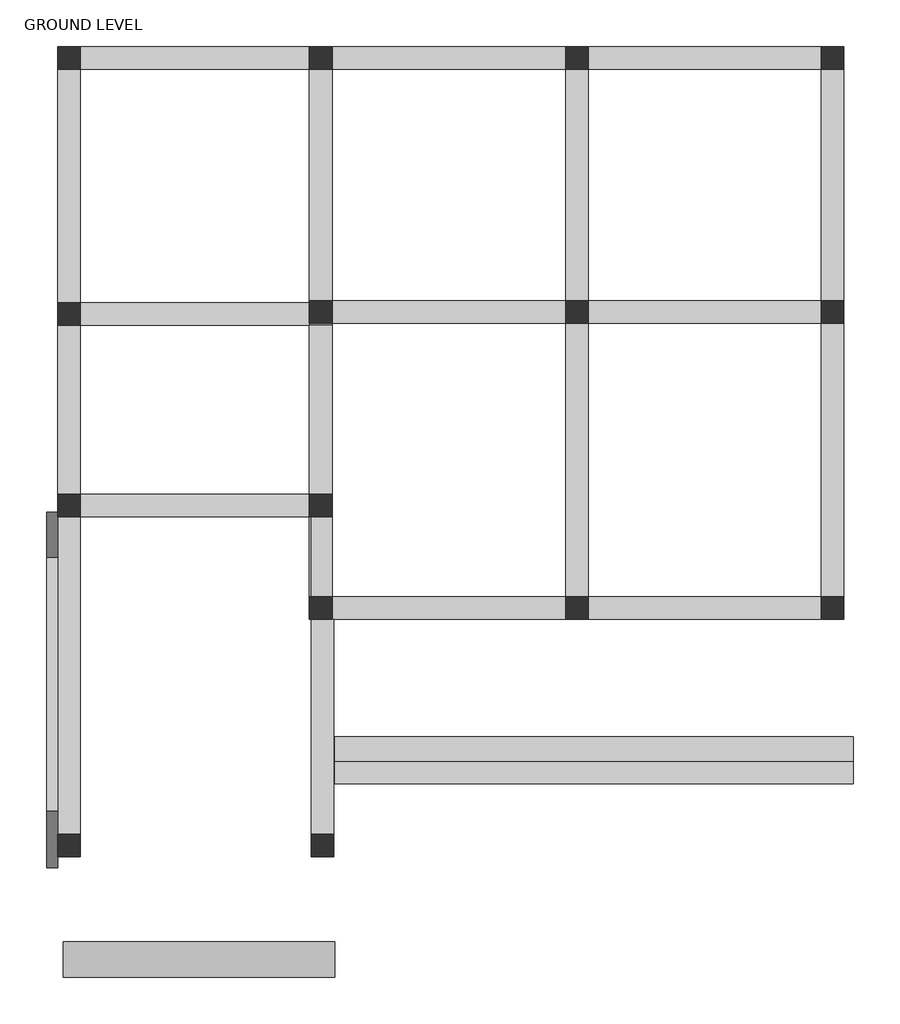
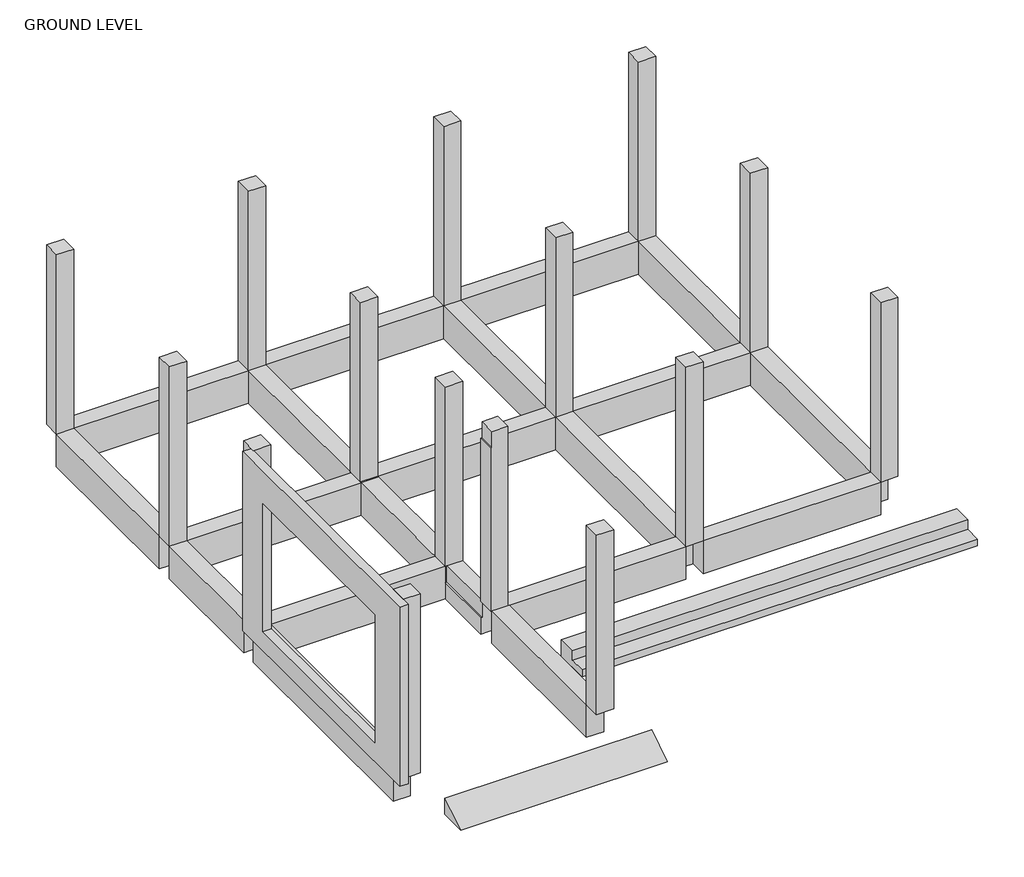
# One storey: 20 beams, 15 columns, 3 proxies.
"""IFC4 building model written with IfcOpenShell, lengths in millimetres."""

from ifc_helpers import new_model, si_unit, frame, origin, origin_with_axes, place, context, project, spatial, polyline, outline, extrude, faceted_brep, transform, mapped, element, save
from components import proxy_c6281e4c, generic_models_12_generic_models_12_89349366, generic_models_13_generic_models_13_4f71b6b5

model = new_model("IFC4")

# Units and contexts
model_context = context("Model", 3, world=origin())
ifc_project = project(units=[si_unit("LENGTHUNIT", "METRE", prefix="MILLI")], contexts=[model_context])

# Site, building, storey
site = spatial("IfcSite", under=ifc_project)
building = spatial("IfcBuilding", under=site)
storey = spatial("IfcBuildingStorey", under=building, Name="GROUND LEVEL", Elevation=0.0)

# Beams
placement = place(None, origin())
element("IfcBeam", 1, ObjectType="Concrete-Rectangular Beam : 12 x 24", at=placement, inside=storey, context=model_context, shape_type="Brep", body=[
    faceted_brep([(-11643.8293601, -6018.4747117, 0.0), (-11339.0293601, -6018.4747117, 0.0), (-11339.0293601, -2868.8747117, 0.0), (-11643.8293601, -2868.8747117, 0.0), (-11643.8293601, -6018.4747117, -609.6), (-11643.8293601, -2868.8747117, -609.6), (-11339.0293601, -6018.4747117, -609.6), (-11339.0293601, -2868.8747117, -609.6), (-11339.0293601, -6018.4747117, -304.8), (-11339.0293601, -2868.8747117, -304.8)], [[[0, 1, 2, 3]], [[4, 0, 3, 5]], [[6, 4, 5, 7]], [[1, 8, 6, 7, 9, 2]], [[2, 9, 7, 5, 3]], [[1, 0, 4, 6, 8]]]),
])
element("IfcBeam", 2, ObjectType="Concrete-Rectangular Beam : 12 x 24", at=placement, inside=storey, context=model_context, shape_type="Brep", body=[
    faceted_brep([(-8251.5270642, -2868.8747117, 0.0), (-8251.5270642, -2564.0747117, 0.0), (-11339.0293601, -2564.0747117, 0.0), (-11339.0293601, -2868.8747117, 0.0), (-8251.5270642, -2868.8747117, -609.6), (-8251.5270642, -2868.8747117, -304.8), (-11339.0293601, -2868.8747117, -304.8), (-11339.0293601, -2868.8747117, -609.6), (-8251.5270642, -2564.0747117, -609.6), (-11339.0293601, -2564.0747117, -609.6)], [[[0, 1, 2, 3]], [[4, 5, 0, 3, 6, 7]], [[8, 4, 7, 9]], [[1, 8, 9, 2]], [[2, 9, 7, 6, 3]], [[1, 0, 5, 4, 8]]]),
])
element("IfcBeam", 3, ObjectType="Concrete-Rectangular Beam : 12 x 24", at=placement, inside=storey, context=model_context, shape_type="Brep", body=[
    faceted_brep([(-4797.1270642, -2868.8747117, 0.0), (-4797.1270642, -2564.0747117, 0.0), (-7946.7270642, -2564.0747117, 0.0), (-7946.7270642, -2868.8747117, 0.0), (-4797.1270642, -2868.8747117, -609.6), (-4797.1270642, -2868.8747117, -304.8), (-7946.7270642, -2868.8747117, -304.8), (-7946.7270642, -2868.8747117, -609.6), (-4797.1270642, -2564.0747117, -609.6), (-7946.7270642, -2564.0747117, -609.6)], [[[0, 1, 2, 3]], [[4, 5, 0, 3, 6, 7]], [[8, 4, 7, 9]], [[1, 8, 9, 2]], [[2, 9, 7, 6, 3]], [[1, 0, 5, 4, 8]]]),
])
element("IfcBeam", 4, ObjectType="Concrete-Rectangular Beam : 12 x 24", at=placement, inside=storey, context=model_context, shape_type="Brep", body=[
    faceted_brep([(-1351.9658472, -2868.8747117, 0.0), (-1351.9658472, -2564.0747117, 0.0), (-4492.3270642, -2564.0747117, 0.0), (-4492.3270642, -2868.8747117, 0.0), (-1351.9658472, -2868.8747117, -609.6), (-1351.9658472, -2868.8747117, -304.8), (-4492.3270642, -2868.8747117, -304.8), (-4492.3270642, -2868.8747117, -609.6), (-1351.9658472, -2564.0747117, -609.6), (-4492.3270642, -2564.0747117, -609.6)], [[[0, 1, 2, 3]], [[4, 5, 0, 3, 6, 7]], [[8, 4, 7, 9]], [[1, 8, 9, 2]], [[2, 9, 7, 6, 3]], [[1, 0, 5, 4, 8]]]),
])
element("IfcBeam", 5, ObjectType="Concrete-Rectangular Beam : 12 x 24", at=placement, inside=storey, context=model_context, shape_type="Brep", body=[
    faceted_brep([(-1351.9658472, -5993.0747117, 0.0), (-1047.1658472, -5993.0747117, 0.0), (-1047.1658472, -2868.8747117, 0.0), (-1351.9658472, -2868.8747117, 0.0), (-1351.9658472, -5993.0747117, -609.6), (-1351.9658472, -5993.0747117, -304.8), (-1351.9658472, -2868.8747117, -304.8), (-1351.9658472, -2868.8747117, -609.6), (-1047.1658472, -5993.0747117, -609.6), (-1047.1658472, -2868.8747117, -609.6)], [[[0, 1, 2, 3]], [[4, 5, 0, 3, 6, 7]], [[8, 4, 7, 9]], [[1, 8, 9, 2]], [[2, 9, 7, 6, 3]], [[1, 0, 5, 4, 8]]]),
])
element("IfcBeam", 6, ObjectType="Concrete-Rectangular Beam : 12 x 24", at=placement, inside=storey, context=model_context, shape_type="Brep", body=[
    faceted_brep([(-7946.7270642, -2868.8747117, 0.0), (-8251.5270642, -2868.8747117, 0.0), (-8251.5270642, -5993.0747117, 0.0), (-7946.7270642, -5993.0747117, 0.0), (-8251.5270642, -2868.8747117, -304.8), (-8251.5270642, -2868.8747117, -609.6), (-8251.5270642, -5993.0747117, -609.6), (-7946.7270642, -2868.8747117, -609.6), (-7946.7270642, -5993.0747117, -609.6), (-7946.7270642, -2868.8747117, -304.8), (-7946.7270642, -5993.0747117, -304.8)], [[[0, 1, 2, 3]], [[1, 4, 5, 6, 2]], [[5, 7, 8, 6]], [[7, 9, 0, 3, 10, 8]], [[0, 9, 7, 5, 4, 1]], [[3, 2, 6, 8, 10]]]),
    faceted_brep([(-7946.7270642, -6323.2747117, 0.0), (-8251.5270642, -6323.2747117, 0.0), (-8251.5270642, -6323.2747117, -609.6), (-7946.7270642, -6323.2747117, -609.6), (-8251.5270642, -6297.8747117, 0.0), (-7946.7270642, -6297.8747117, 0.0), (-7946.7270642, -6297.8747117, -609.6), (-8251.5270642, -6297.8747117, -609.6)], [[[0, 1, 2, 3]], [[4, 5, 6, 7]], [[1, 0, 5, 4]], [[2, 1, 4, 7]], [[3, 2, 7, 6]], [[0, 3, 6, 5]]]),
])
element("IfcBeam", 7, ObjectType="Concrete-Rectangular Beam : 12 x 24", at=placement, inside=storey, context=model_context, shape_type="Brep", body=[
    faceted_brep([(-1351.9658472, -9984.0050402, 0.0), (-1047.1658472, -9984.0050402, 0.0), (-1047.1658472, -6297.8747117, 0.0), (-1351.9658472, -6297.8747117, 0.0), (-1351.9658472, -9984.0050402, -609.6), (-1351.9658472, -9984.0050402, -304.8), (-1351.9658472, -6297.8747117, -304.8), (-1351.9658472, -6297.8747117, -609.6), (-1047.1658472, -9984.0050402, -609.6), (-1047.1658472, -6297.8747117, -609.6)], [[[0, 1, 2, 3]], [[4, 5, 0, 3, 6, 7]], [[8, 4, 7, 9]], [[1, 8, 9, 2]], [[2, 9, 7, 6, 3]], [[1, 0, 5, 4, 8]]]),
])
element("IfcBeam", 8, ObjectType="Concrete-Rectangular Beam : 12 x 24", at=placement, inside=storey, context=model_context, shape_type="Brep", body=[
    faceted_brep([(-4492.3270642, -9984.0050402, 0.0), (-4492.3270642, -10288.8050402, 0.0), (-1351.9658472, -10288.8050402, 0.0), (-1351.9658472, -9984.0050402, 0.0), (-4492.3270642, -9984.0050402, -609.6), (-4492.3270642, -9984.0050402, -304.8), (-1351.9658472, -9984.0050402, -304.8), (-1351.9658472, -9984.0050402, -609.6), (-4492.3270642, -10288.8050402, -609.6), (-1351.9658472, -10288.8050402, -609.6)], [[[0, 1, 2, 3]], [[4, 5, 0, 3, 6, 7]], [[8, 4, 7, 9]], [[1, 8, 9, 2]], [[1, 0, 5, 4, 8]], [[2, 9, 7, 6, 3]]]),
])
element("IfcBeam", 9, ObjectType="Concrete-Rectangular Beam : 12 x 24", at=placement, inside=storey, context=model_context, shape_type="Brep", body=[
    faceted_brep([(-7946.7270642, -9984.0050402, 0.0), (-7946.7270642, -10288.8050402, 0.0), (-7921.3270642, -10288.8050402, 0.0), (-4797.1270642, -10288.8050402, 0.0), (-4797.1270642, -9984.0050402, 0.0), (-4801.7464557, -9984.0050402, 0.0), (-7942.1076727, -9984.0050402, 0.0), (-7946.7270642, -9984.0050402, -609.6), (-4797.1270642, -9984.0050402, -609.6), (-7946.7270642, -10288.8050402, -609.6), (-4797.1270642, -10288.8050402, -609.6), (-7921.3270642, -10288.8050402, -609.6)], [[[0, 1, 2, 3, 4, 5, 6]], [[7, 0, 6, 5, 4, 8]], [[9, 7, 8, 10, 11]], [[1, 9, 11, 10, 3, 2]], [[1, 0, 7, 9]], [[3, 10, 8, 4]]]),
])
element("IfcBeam", 10, ObjectType="Concrete-Rectangular Beam : 12 x 24", at=placement, inside=storey, context=model_context, shape_type="SweptSolid", body=[
    extrude(outline(polyline([(-609.6, -8251.5270642), (-609.6, -7946.7270642), (0.0, -7946.7270642), (0.0, -8226.1270642), (-304.8, -8226.1270642), (-304.8, -8251.5270642), (-609.6, -8251.5270642)])), frame((0.0, -9984.0050402, 0.0), z_axis=(0.0, 1.0, 0.0), x_axis=(0.0, 0.0, 1.0)), (0.0, 0.0, 1.0), 1081.2677011),
])
element("IfcBeam", 11, ObjectType="Concrete-Rectangular Beam : 12 x 24", at=placement, inside=storey, context=model_context, shape_type="Brep", body=[
    faceted_brep([(-8251.5270642, -8597.9373391, 0.0), (-7946.7270642, -8597.9373391, 0.0), (-7946.7270642, -6323.2747117, 0.0), (-8251.5270642, -6323.2747117, 0.0), (-8251.5270642, -7013.8396616, 0.0), (-8251.5270642, -7547.2396616, 0.0), (-8251.5270642, -8461.6396616, 0.0), (-7946.7270642, -8597.9373391, -609.6), (-7946.7270642, -6323.2747117, -609.6), (-8251.5270642, -8597.9373391, -609.6), (-8251.5270642, -6323.2747117, -609.6), (-8251.5270642, -8597.9373391, -304.8)], [[[0, 1, 2, 3, 4, 5, 6]], [[1, 7, 8, 2]], [[7, 9, 10, 8]], [[9, 11, 0, 6, 5, 4, 3, 10]], [[0, 11, 9, 7, 1]], [[3, 2, 8, 10]]]),
])
element("IfcBeam", 12, ObjectType="Concrete-Rectangular Beam : 12 x 24", at=placement, inside=storey, context=model_context, shape_type="Brep", body=[
    faceted_brep([(-11339.0293601, -8597.9373391, 0.0), (-11339.0293601, -8902.7373391, 0.0), (-8251.5270642, -8902.7373391, 0.0), (-8251.5270642, -8597.9373391, 0.0), (-11339.0293601, -8597.9373391, -609.6), (-11339.0293601, -8597.9373391, -304.8), (-8251.5270642, -8597.9373391, -609.6), (-11339.0293601, -8902.7373391, -609.6), (-8251.5270642, -8902.7373391, -609.6), (-11339.0293601, -8902.7373391, -304.8)], [[[0, 1, 2, 3]], [[4, 5, 0, 3, 6]], [[7, 4, 6, 8]], [[1, 9, 7, 8, 2]], [[1, 0, 5, 4, 7, 9]], [[2, 8, 6, 3]]]),
])
element("IfcBeam", 13, ObjectType="Concrete-Rectangular Beam : 12 x 24", at=placement, inside=storey, context=model_context, shape_type="Brep", body=[
    faceted_brep([(-11339.0293601, -6323.2747117, 0.0), (-11643.8293601, -6323.2747117, 0.0), (-11643.8293601, -8597.9373391, 0.0), (-11339.0293601, -8597.9373391, 0.0), (-11339.0293601, -6323.2747117, -609.6), (-11339.0293601, -6323.2747117, -304.8), (-11339.0293601, -8597.9373391, -304.8), (-11339.0293601, -8597.9373391, -609.6), (-11643.8293601, -6323.2747117, -609.6), (-11643.8293601, -8597.9373391, -609.6)], [[[0, 1, 2, 3]], [[4, 5, 0, 3, 6, 7]], [[8, 4, 7, 9]], [[1, 8, 9, 2]], [[1, 0, 5, 4, 8]], [[2, 9, 7, 6, 3]]]),
])
element("IfcBeam", 14, ObjectType="Concrete-Rectangular Beam : 12 x 24", at=placement, inside=storey, context=model_context, shape_type="Brep", body=[
    faceted_brep([(-8251.5270642, -6018.4747117, 0.0), (-8251.5270642, -6297.8747117, 0.0), (-8251.5270642, -6323.2747117, 0.0), (-8251.5270642, -6323.2747117, -609.6), (-8251.5270642, -6297.8747117, -609.6), (-8251.5270642, -6018.4747117, -609.6), (-8251.5270642, -6018.4747117, -304.8), (-11339.0293601, -6018.4747117, 0.0), (-11339.0293601, -6323.2747117, 0.0), (-11264.7236584, -6323.2747117, 0.0), (-11339.0293601, -6323.2747117, -304.8), (-11339.0293601, -6323.2747117, -609.6), (-11339.0293601, -6018.4747117, -609.6), (-11339.0293601, -6018.4747117, -304.8)], [[[0, 1, 2, 3, 4, 5, 6]], [[2, 1, 0, 7, 8, 9]], [[3, 2, 9, 8, 10, 11]], [[5, 4, 3, 11, 12]], [[0, 6, 5, 12, 13, 7]], [[7, 13, 12, 11, 10, 8]]]),
])
element("IfcBeam", 15, ObjectType="Concrete-Rectangular Beam : 12 x 24", at=placement, inside=storey, context=model_context, shape_type="Brep", body=[
    faceted_brep([(-4492.3270642, -6297.8747117, 0.0), (-4797.1270642, -6297.8747117, 0.0), (-4797.1270642, -9984.0050402, 0.0), (-4492.3270642, -9984.0050402, 0.0), (-4492.3270642, -6297.8747117, -609.6), (-4492.3270642, -6297.8747117, -304.8), (-4492.3270642, -9984.0050402, -304.8), (-4492.3270642, -9984.0050402, -609.6), (-4797.1270642, -6297.8747117, -609.6), (-4797.1270642, -9984.0050402, -609.6)], [[[0, 1, 2, 3]], [[4, 5, 0, 3, 6, 7]], [[8, 4, 7, 9]], [[1, 8, 9, 2]], [[1, 0, 5, 4, 8]], [[2, 9, 7, 6, 3]]]),
])
element("IfcBeam", 16, ObjectType="Concrete-Rectangular Beam : 12 x 24", at=placement, inside=storey, context=model_context, shape_type="Brep", body=[
    faceted_brep([(-4492.3270642, -5993.0747117, 0.0), (-4492.3270642, -6297.8747117, 0.0), (-1351.9658472, -6297.8747117, 0.0), (-1351.9658472, -5993.0747117, 0.0), (-4492.3270642, -5993.0747117, -609.6), (-4492.3270642, -5993.0747117, -304.8), (-1351.9658472, -5993.0747117, -304.8), (-1351.9658472, -5993.0747117, -609.6), (-4492.3270642, -6297.8747117, -609.6), (-1351.9658472, -6297.8747117, -609.6), (-4492.3270642, -6297.8747117, -304.8), (-1351.9658472, -6297.8747117, -304.8)], [[[0, 1, 2, 3]], [[4, 5, 0, 3, 6, 7]], [[8, 4, 7, 9]], [[1, 10, 8, 9, 11, 2]], [[2, 11, 9, 7, 6, 3]], [[1, 0, 5, 4, 8, 10]]]),
])
element("IfcBeam", 17, ObjectType="Concrete-Rectangular Beam : 12 x 24", at=placement, inside=storey, context=model_context, shape_type="Brep", body=[
    faceted_brep([(-4492.3270642, -2868.8747117, 0.0), (-4797.1270642, -2868.8747117, 0.0), (-4797.1270642, -5993.0747117, 0.0), (-4492.3270642, -5993.0747117, 0.0), (-4492.3270642, -2868.8747117, -609.6), (-4492.3270642, -2868.8747117, -304.8), (-4492.3270642, -5993.0747117, -304.8), (-4492.3270642, -5993.0747117, -609.6), (-4797.1270642, -2868.8747117, -609.6), (-4797.1270642, -5993.0747117, -609.6), (-4797.1270642, -2868.8747117, -304.8), (-4797.1270642, -5993.0747117, -304.8)], [[[0, 1, 2, 3]], [[4, 5, 0, 3, 6, 7]], [[8, 4, 7, 9]], [[1, 10, 8, 9, 11, 2]], [[1, 0, 5, 4, 8, 10]], [[2, 11, 9, 7, 6, 3]]]),
])
element("IfcBeam", 18, ObjectType="Concrete-Rectangular Beam : 12 x 24", at=placement, inside=storey, context=model_context, shape_type="Brep", body=[
    faceted_brep([(-4797.1270642, -6297.8747117, 0.0), (-4797.1270642, -5993.0747117, 0.0), (-7946.7270642, -5993.0747117, 0.0), (-7946.7270642, -6297.8747117, 0.0), (-7889.5770642, -6297.8747117, 0.0), (-4801.7464557, -6297.8747117, 0.0), (-4797.1270642, -6297.8747117, -609.6), (-7946.7270642, -6297.8747117, -609.6), (-4797.1270642, -5993.0747117, -609.6), (-7946.7270642, -5993.0747117, -609.6), (-4797.1270642, -5993.0747117, -304.8), (-7946.7270642, -5993.0747117, -304.8)], [[[0, 1, 2, 3, 4, 5]], [[6, 0, 5, 4, 3, 7]], [[8, 6, 7, 9]], [[1, 10, 8, 9, 11, 2]], [[1, 0, 6, 8, 10]], [[3, 2, 11, 9, 7]]]),
])
element("IfcBeam", 19, ObjectType="Concrete-Rectangular Beam : 12 x 24", at=placement, inside=storey, context=model_context, shape_type="Brep", body=[
    faceted_brep([(-11339.0293601, -8902.7373391, 0.0), (-11643.8293601, -8902.7373391, 0.0), (-11643.8293601, -13183.002305, 0.0), (-11339.0293601, -13183.002305, 0.0), (-11339.0293601, -8902.7373391, -609.6), (-11339.0293601, -13183.002305, -304.8), (-11339.0293601, -13183.002305, -609.6), (-11643.8293601, -8902.7373391, -609.6), (-11643.8293601, -13183.002305, -609.6)], [[[0, 1, 2, 3]], [[4, 0, 3, 5, 6]], [[7, 4, 6, 8]], [[1, 7, 8, 2]], [[1, 0, 4, 7]], [[2, 8, 6, 5, 3]]]),
])
element("IfcBeam", 20, ObjectType="Concrete-Rectangular Beam : 12 x 24", at=placement, inside=storey, context=model_context, shape_type="Brep", body=[
    faceted_brep([(-7921.3270642, -10288.8050402, 0.0), (-7946.7270642, -10288.8050402, 0.0), (-8226.1270642, -10288.8050402, 0.0), (-8226.1270642, -13183.002305, 0.0), (-7921.3270642, -13183.002305, 0.0), (-8226.1270642, -10288.8050402, -609.6), (-8226.1270642, -13183.002305, -609.6), (-8226.1270642, -13183.002305, -304.8), (-7946.7270642, -10288.8050402, -609.6), (-7921.3270642, -10288.8050402, -609.6), (-7921.3270642, -13183.002305, -609.6)], [[[0, 1, 2, 3, 4]], [[2, 5, 6, 7, 3]], [[5, 8, 9, 10, 6]], [[9, 0, 4, 10]], [[0, 9, 8, 5, 2, 1]], [[4, 3, 7, 6, 10]]]),
])

# Proxies
proxy_shape = proxy_c6281e4c(model_context)
element("IfcBuildingElementProxy", 21, Name="GENERIC WALL 6\" : GENERIC WALL 6\"", ObjectType="GENERIC WALL 6\" : GENERIC WALL 6\"", at=placement, inside=storey, context=model_context, shape_type="MappedRepresentation", body=[
    mapped(proxy_shape, transform((0.0, 0.0, 0.0), x_axis=(1.0, 0.0, 0.0), y_axis=(0.0, 1.0, 0.0), z_axis=(0.0, 0.0, 1.0))),
])
generic_models_12_generic_models_12_shape = generic_models_12_generic_models_12_89349366(model_context)
element("IfcBuildingElementProxy", 22, Name="Generic Models 12 : Generic Models 12", ObjectType="Generic Models 12 : Generic Models 12", at=placement, inside=storey, context=model_context, shape_type="MappedRepresentation", body=[
    mapped(generic_models_12_generic_models_12_shape, transform((0.0, 0.0, 0.0), x_axis=(1.0, 0.0, 0.0), y_axis=(0.0, 1.0, 0.0), z_axis=(0.0, 0.0, 1.0))),
])
generic_models_13_generic_models_13_shape = generic_models_13_generic_models_13_4f71b6b5(model_context)
element("IfcBuildingElementProxy", 23, Name="Generic Models 13 : Generic Models 13", ObjectType="Generic Models 13 : Generic Models 13", at=placement, inside=storey, context=model_context, shape_type="MappedRepresentation", body=[
    mapped(generic_models_13_generic_models_13_shape, transform((0.0, 0.0, 0.0), x_axis=(1.0, 0.0, 0.0), y_axis=(0.0, 1.0, 0.0), z_axis=(0.0, 0.0, 1.0))),
])

# Columns
element("IfcColumn", 24, ObjectType="Concrete-Rectangular-Column : 12\" X 12\" COLUMN", at=placement, inside=storey, context=model_context, shape_type="SweptSolid", body=[
    extrude(outline(polyline([(-11339.0293601, -2564.0747117), (-11339.0293601, -2868.8747117), (-11643.8293601, -2868.8747117), (-11643.8293601, -2564.0747117), (-11339.0293601, -2564.0747117)])), origin_with_axes(), (0.0, 0.0, 1.0), 3352.8),
])
element("IfcColumn", 25, ObjectType="Concrete-Rectangular-Column : 12\" X 12\" COLUMN", at=placement, inside=storey, context=model_context, shape_type="SweptSolid", body=[
    extrude(outline(polyline([(-7946.7270642, -2564.0747117), (-7946.7270642, -2868.8747117), (-8251.5270642, -2868.8747117), (-8251.5270642, -2564.0747117), (-7946.7270642, -2564.0747117)])), origin_with_axes(), (0.0, 0.0, 1.0), 3352.8),
])
element("IfcColumn", 26, ObjectType="Concrete-Rectangular-Column : 12\" X 12\" COLUMN", at=placement, inside=storey, context=model_context, shape_type="SweptSolid", body=[
    extrude(outline(polyline([(-4492.3270642, -2564.0747117), (-4492.3270642, -2868.8747117), (-4797.1270642, -2868.8747117), (-4797.1270642, -2564.0747117), (-4492.3270642, -2564.0747117)])), origin_with_axes(), (0.0, 0.0, 1.0), 3352.8),
])
element("IfcColumn", 27, ObjectType="Concrete-Rectangular-Column : 12\" X 12\" COLUMN", at=placement, inside=storey, context=model_context, shape_type="SweptSolid", body=[
    extrude(outline(polyline([(-1047.1658472, -2564.0747117), (-1047.1658472, -2868.8747117), (-1351.9658472, -2868.8747117), (-1351.9658472, -2564.0747117), (-1047.1658472, -2564.0747117)])), origin_with_axes(), (0.0, 0.0, 1.0), 3352.8),
])
element("IfcColumn", 28, ObjectType="Concrete-Rectangular-Column : 12\" X 12\" COLUMN", at=placement, inside=storey, context=model_context, shape_type="SweptSolid", body=[
    extrude(outline(polyline([(-1047.1658472, -5993.0747117), (-1047.1658472, -6297.8747117), (-1351.9658472, -6297.8747117), (-1351.9658472, -5993.0747117), (-1047.1658472, -5993.0747117)])), origin_with_axes(), (0.0, 0.0, 1.0), 3352.8),
])
element("IfcColumn", 29, ObjectType="Concrete-Rectangular-Column : 12\" X 12\" COLUMN", at=placement, inside=storey, context=model_context, shape_type="SweptSolid", body=[
    extrude(outline(polyline([(-4492.3270642, -5993.0747117), (-4492.3270642, -6297.8747117), (-4797.1270642, -6297.8747117), (-4797.1270642, -5993.0747117), (-4492.3270642, -5993.0747117)])), origin_with_axes(), (0.0, 0.0, 1.0), 3352.8),
])
element("IfcColumn", 30, ObjectType="Concrete-Rectangular-Column : 12\" X 12\" COLUMN", at=placement, inside=storey, context=model_context, shape_type="Brep", body=[
    faceted_brep([(-7946.7270642, -5993.0747117, 0.0), (-7946.7270642, -6297.8747117, 0.0), (-8251.5270642, -6297.8747117, 0.0), (-8251.5270642, -5993.0747117, 0.0), (-7946.7270642, -5993.0747117, 3352.8), (-7946.7270642, -6297.8747117, 3352.8), (-8251.5270642, -6297.8747117, 3352.8), (-8251.5270642, -6018.4747117, 3352.8), (-8251.5270642, -5993.0747117, 3352.8)], [[[0, 1, 2, 3]], [[4, 5, 1, 0]], [[5, 6, 2, 1]], [[6, 7, 8, 3, 2]], [[8, 4, 0, 3]], [[4, 8, 7, 6, 5]]]),
])
element("IfcColumn", 31, ObjectType="Concrete-Rectangular-Column : 12\" X 12\" COLUMN", at=placement, inside=storey, context=model_context, shape_type="SweptSolid", body=[
    extrude(outline(polyline([(-11339.0293601, -6018.4747117), (-11339.0293601, -6323.2747117), (-11643.8293601, -6323.2747117), (-11643.8293601, -6018.4747117), (-11339.0293601, -6018.4747117)])), origin_with_axes(), (0.0, 0.0, 1.0), 3352.8),
])
element("IfcColumn", 32, ObjectType="Concrete-Rectangular-Column : 12\" X 12\" COLUMN", at=placement, inside=storey, context=model_context, shape_type="SweptSolid", body=[
    extrude(outline(polyline([(-11339.0293601, -8597.9373391), (-11339.0293601, -8902.7373391), (-11643.8293601, -8902.7373391), (-11643.8293601, -8597.9373391), (-11339.0293601, -8597.9373391)])), origin_with_axes(), (0.0, 0.0, 1.0), 3352.8),
])
element("IfcColumn", 33, ObjectType="Concrete-Rectangular-Column : 12\" X 12\" COLUMN", at=placement, inside=storey, context=model_context, shape_type="SweptSolid", body=[
    extrude(outline(polyline([(-7946.7270642, -8597.9373391), (-7946.7270642, -8902.7373391), (-8251.5270642, -8902.7373391), (-8251.5270642, -8597.9373391), (-7946.7270642, -8597.9373391)])), origin_with_axes(), (0.0, 0.0, 1.0), 3352.8),
])
element("IfcColumn", 34, ObjectType="Concrete-Rectangular-Column : 12\" X 12\" COLUMN", at=placement, inside=storey, context=model_context, shape_type="SweptSolid", body=[
    extrude(outline(polyline([(-7921.3270642, -13183.002305), (-7921.3270642, -13487.802305), (-8226.1270642, -13487.802305), (-8226.1270642, -13183.002305), (-7921.3270642, -13183.002305)])), origin_with_axes(), (0.0, 0.0, 1.0), 3352.8),
])
element("IfcColumn", 35, ObjectType="Concrete-Rectangular-Column : 12\" X 12\" COLUMN", at=placement, inside=storey, context=model_context, shape_type="SweptSolid", body=[
    extrude(outline(polyline([(-11339.0293601, -13183.002305), (-11339.0293601, -13487.802305), (-11643.8293601, -13487.802305), (-11643.8293601, -13183.002305), (-11339.0293601, -13183.002305)])), origin_with_axes(), (0.0, 0.0, 1.0), 3352.8),
])
element("IfcColumn", 36, ObjectType="Concrete-Rectangular-Column : 12\" X 12\" COLUMN", at=placement, inside=storey, context=model_context, shape_type="SweptSolid", body=[
    extrude(outline(polyline([(0.0, -8251.5270642), (0.0, -7946.7270642), (3352.8, -7946.7270642), (3352.8, -8226.1270642), (3048.0, -8226.1270642), (3048.0, -8251.5270642), (0.0, -8251.5270642)])), frame((0.0, -10288.8050402, 0.0), z_axis=(0.0, 1.0, 0.0), x_axis=(0.0, 0.0, 1.0)), (0.0, 0.0, 1.0), 304.8),
])
element("IfcColumn", 37, ObjectType="Concrete-Rectangular-Column : 12\" X 12\" COLUMN", at=placement, inside=storey, context=model_context, shape_type="SweptSolid", body=[
    extrude(outline(polyline([(-4492.3270642, -9984.0050402), (-4492.3270642, -10288.8050402), (-4797.1270642, -10288.8050402), (-4797.1270642, -9984.0050402), (-4492.3270642, -9984.0050402)])), origin_with_axes(), (0.0, 0.0, 1.0), 3352.8),
])
element("IfcColumn", 38, ObjectType="Concrete-Rectangular-Column : 12\" X 12\" COLUMN", at=placement, inside=storey, context=model_context, shape_type="SweptSolid", body=[
    extrude(outline(polyline([(-1047.1658472, -9984.0050402), (-1047.1658472, -10288.8050402), (-1351.9658472, -10288.8050402), (-1351.9658472, -9984.0050402), (-1047.1658472, -9984.0050402)])), origin_with_axes(), (0.0, 0.0, 1.0), 3352.8),
])

save(model, "model.ifc")

# Revit data of these elements
# Type "Concrete-Rectangular Beam : 12 x 24"
#   Assembly Code = "B10"
#   Length [instance default] = 5' - 0"
#   b = 1' - 0"
#   h = 2' - 0"
#   Structural Material [instance default] = Concrete, Cast-in-Place gray
# Type "Concrete-Rectangular-Column : 12\" X 12\" COLUMN"
#   Assembly Code = "B10"
#   b = 1' - 0"
#   h = 1' - 0"
#   Structural Material [instance default] = Concrete, Cast-in-Place gray
# Elements 1, 2, 3, 4, 5, 6, 7, 8, 9, 10, 11, 12, 13, 14, 15, 16, 17, 18, 19, 20 (IfcBeam, "Concrete-Rectangular Beam : 12 x 24")
#   Structural Material = Concrete, Cast-in-Place gray
#   Phase Created = New Construction
#   Materials on its faces: "Concrete, Cast-in-Place gray"
# Element 21 (IfcBuildingElementProxy, "GENERIC WALL 6\" : GENERIC WALL 6\"")
#   Phase Created = New Construction
#   Materials on its faces: "ACCENT BEIGE COLOUR"
# Element 22 (IfcBuildingElementProxy, "Generic Models 12 : Generic Models 12")
#   Phase Created = New Construction
#   Materials on its faces: "Concrete, Cast-in-Place gray"
# Element 23 (IfcBuildingElementProxy, "Generic Models 13 : Generic Models 13")
#   Phase Created = New Construction
#   Materials on its faces: "Concrete, Cast-in-Place gray"
# Elements 24, 25, 26, 27, 28, 32, 33, 34, 36, 37, 38 (IfcColumn, "Concrete-Rectangular-Column : 12\" X 12\" COLUMN")
#   Structural Material = Concrete, Cast-in-Place gray
#   Phase Created = New Construction
#   Materials on its faces: "Concrete, Cast-in-Place gray", "beige colour"
# Elements 29, 30, 31 (IfcColumn, "Concrete-Rectangular-Column : 12\" X 12\" COLUMN")
#   Structural Material = Concrete, Cast-in-Place gray
#   Phase Created = New Construction
#   Materials on its faces: "Concrete, Cast-in-Place gray"
# Element 35 (IfcColumn, "Concrete-Rectangular-Column : 12\" X 12\" COLUMN")
#   Structural Material = Concrete, Cast-in-Place gray
#   Phase Created = New Construction
#   Materials on its faces: "beige colour", "Concrete, Cast-in-Place gray"
# Materials
#   "Concrete, Cast-in-Place gray": class "Concrete", colour RGB 192 192 192, transparency 0, Description = "Cast-in-place concrete", Cost = 0
#   "ACCENT BEIGE COLOUR": class "Generic", colour RGB 120 120 120, transparency 0, Cost = 0
#   "beige colour": class "Generic", colour RGB 120 120 120, transparency 0, Cost = 0
